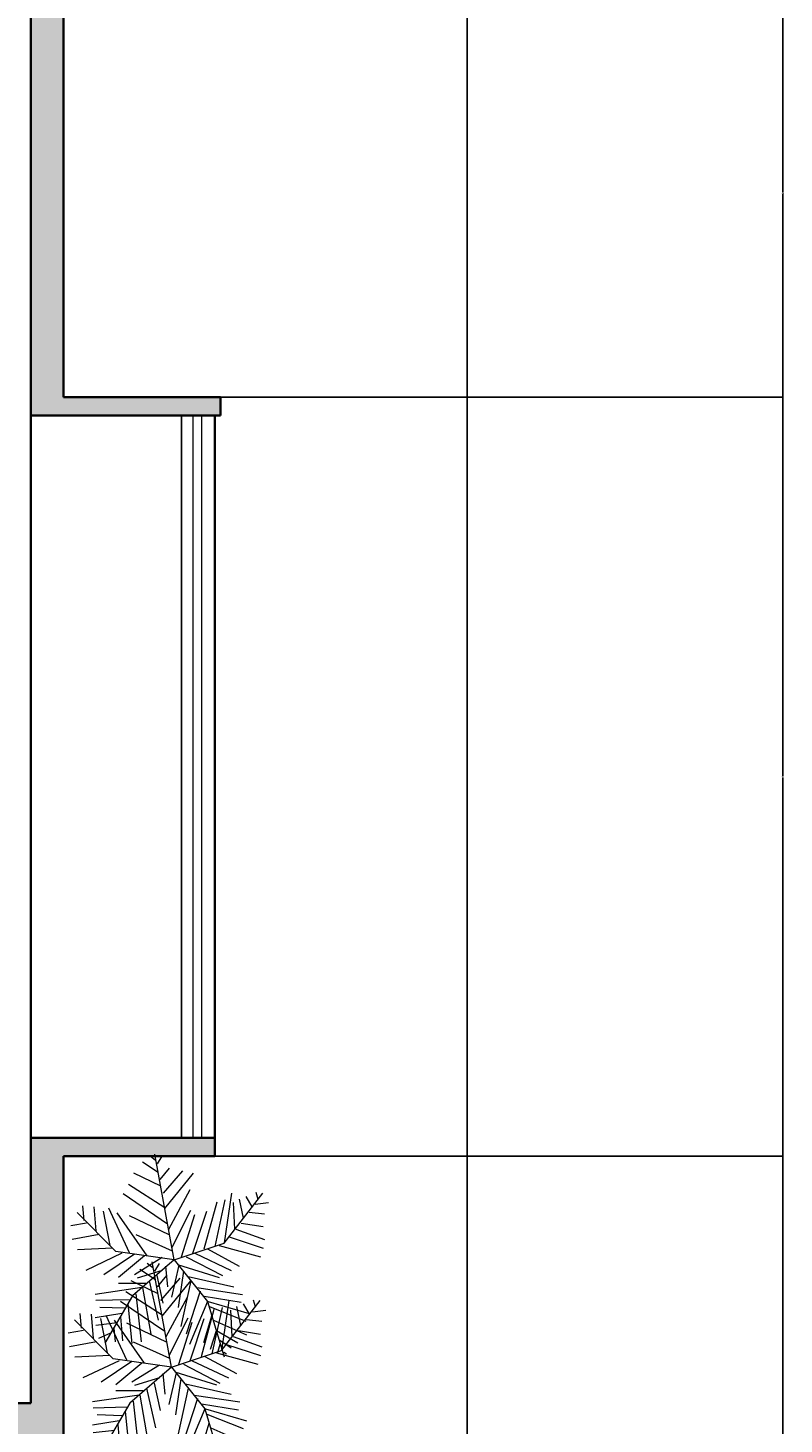
# Model space of a CAD drawing. Units: inches. Extents: x 192 to 1361, y -1362 to 367.
# Tile 22 of 23: x 1153 to 1361, y -454 to -71. Entities that reach past the tile are written whole.
import ezdxf

# ---------------------------------------------------------------- set-up
doc = ezdxf.new("R2010")
doc.units = ezdxf.units.IN
doc.header["$MEASUREMENT"] = 0
for name, color, linetype, lineweight in [('A-ANNO-DIMS', 2, 'Continuous', 18), ('A-WALL-PATT', 250, 'Continuous', 13), ('lawn', 96, 'Continuous', 13), ('walls', 7, 'Continuous', 35), ('windows', 4, 'Continuous', 18)]:
    doc.layers.add(name, color=color, linetype=linetype, lineweight=lineweight)
doc.styles.get("Standard").update_dxf_attribs({"font": 'arial.ttf'})
doc.dimstyles.get("Standard").update_dxf_attribs({"dimtxt": 0.18, "dimasz": 0.18, "dimexe": 0.18, "dimexo": 0.0625, "dimgap": 0.09, "dimtad": 0, "dimtih": 1, "dimtoh": 1, "dimzin": 0, "dimdsep": 46, "dimlunit": 3, "dimtxsty": 'Standard', "dimcen": 0.09, "dimadec": 0, "dimazin": 0, "dimtfac": 1, "dimtofl": 0, "dimtmove": 0, "dimatfit": 3, "dimfxl": 1, "dimtolj": 1, "dimtzin": 0, "dimarcsym": 0})

# ---------------------------------------------------------------- blocks, each defined once
blk = doc.blocks.new('*U4')
for p, q in [((-10.186, 53.64), (-13.084, 55.962)), ((0, 0), (-10.5, 57)), ((-9.099, 51.782), (-6.563, 55.962)), ((-7.288, 39.707), (-21.778, 46.673)), ((-8.737, 47.138), (-17.069, 52.711)), ((-7.65, 43.423), (-2.578, 49.46)), ((-5.839, 35.992), (4.667, 48.067)), ((-5.114, 27.632), (10.463, 46.673)), ((-5.114, 28.097), (-24.676, 40.636)), ((-2.941, 16.486), (8.652, 37.85)), ((-3.665, 19.273), (-27.574, 35.527)), ((16.259, 5.805), (23.142, 31.348)), ((22.055, 7.198), (27.489, 32.277)), ((27, 9), (48, 36)), ((27.127, 9.056), (31.112, 35.992)), ((31.836, 30.883), (32.561, 16.486)), ((35.096, 32.741), (37.27, 22.524)), ((38.719, 34.134), (41.979, 28.561)), ((43.791, 29.954), (51.036, 30.883)), ((44.153, 36.456), (45.239, 32.741)), ((-31.5, 4.5), (-52.5, 25.5)), ((-48.585, 21.131), (-49.309, 29.026)), ((-43.513, 28.561), (-42.427, 15.558)), ((-38.442, 26.239), (-34.819, 7.663)), ((-35.544, 28.097), (-24.314, 3.947)), ((-14.533, 2.09), (-30.834, 25.31)), ((-24.314, 23.917), (-2.941, 13.7)), ((-1.129, 6.734), (9.014, 26.704)), ((3.942, 1.625), (11.187, 24.381)), ((10.101, 3.483), (17.708, 26.239)), ((40.53, 25.775), (48.862, 24.846)), ((-47.498, 19.737), (-55.83, 18.344)), ((33.285, 16.486), (48.862, 10.913)), ((36.183, 19.737), (48.137, 17.88)), ((-40.615, 13.7), (-55.105, 10.913)), ((-20.691, 13.7), (-1.129, 4.876)), ((0, 0), (27, 9)), ((24.229, 7.663), (46.688, 1.625)), ((29.662, 12.307), (48.137, 6.269)), ((-33.37, 6.269), (-52.207, 5.34)), ((-28.299, 3.483), (-47.86, -5.805)), ((-21.416, 3.018), (-38.079, -8.128)), ((0, 0), (-31.5, 4.5)), ((-15.982, 2.09), (-30.11, -9.521)), ((0, 0), (-22.5, -19.5)), ((-6.563, 1.161), (-21.416, -8.128)), ((0, 0), (18, -22.5)), ((6.478, 1.625), (26.04, -8.592)), ((11.187, 3.483), (30.749, -5.805)), ((18.07, 5.805), (35.096, -3.483)), ((-6.563, -5.805), (-19.967, -9.985)), ((-4.752, -3.483), (-3.665, -14.629)), ((2.493, -3.019), (-1.491, -20.202)), ((1.769, -2.555), (24.229, -9.521)), ((5.029, -6.27), (2.131, -25.775)), ((-15.257, -12.772), (-30.11, -12.772)), ((-13.446, -11.378), (-8.737, -32.741)), ((-9.461, -8.592), (-6.201, -23.453)), ((9.014, -11.378), (3.58, -35.992)), ((7.565, -9.056), (32.198, -14.629)), ((-17.431, -15.094), (-42.789, -18.809)), ((-24.314, -21.596), (-42.427, -22.06)), ((-22.5, -19.5), (-37.5, -45)), ((-20.691, -18.345), (-17.793, -44.352)), ((-17.069, -15.094), (-12.721, -40.172)), ((14.085, -16.951), (6.478, -40.172)), ((18.07, -22.524), (8.289, -45.745)), ((12.274, -15.094), (36.907, -18.809)), ((16.259, -19.738), (36.183, -22.989)), ((18, -22.5), (27, -52.5)), ((18.433, -22.524), (40.53, -29.026)), ((-28.299, -29.026), (-42.789, -31.348)), ((-26.849, -26.24), (-40.253, -25.775)), ((-25.038, -23.918), (-22.865, -45.281)), ((19.157, -25.311), (38.719, -33.206)), ((-30.834, -34.135), (-42.427, -35.528)), ((-32.646, -36.921), (-31.921, -44.352)), ((-29.023, -30.884), (-27.936, -43.887)), ((20.244, -30.419), (15.897, -44.816)), ((21.331, -32.741), (39.081, -40.636)), ((-34.457, -39.708), (-40.978, -42.494)), ((22.78, -37.85), (19.519, -48.532)), ((22.78, -38.314), (34.372, -44.816)), ((24.591, -43.423), (30.749, -47.603)), ((24.591, -45.745), (23.142, -50.854)), ((26.764, -49.925), (28.213, -50.854))]:
    blk.add_line(p, q)
blk = doc.blocks.new('*D52')
at = {"layer": 'A-ANNO-DIMS', "color": 0, "lineweight": -2, "transparency": 16777216}
for p, q in [((1162.8, -60.44), (1162.8, 367.39)), ((1162.98, 367.21), (1217.73, 367.21)), ((1273.39, 367.21), (1218.64, 367.21)), ((1273.57, -597.44), (1273.57, 367.39))]:
    blk.add_line(p, q, dxfattribs=at)
at = {"layer": 'A-ANNO-DIMS', "color": 0, "transparency": 16777216}
for points in [[(1162.98, 367.24), (1162.98, 367.18), (1162.8, 367.21)], [(1273.39, 367.24), (1273.39, 367.18), (1273.57, 367.21)]]:
    blk.add_solid(points, dxfattribs=at)
at = {"layer": 'Defpoints', "color": 0, "transparency": 16777216}
for p in [(1273.57, 367.21), (1162.8, -60.5), (1273.57, -597.5)]:
    blk.add_point(p, dxfattribs=at)
at = {"layer": 'A-ANNO-DIMS', "color": 0, "transparency": 16777216, "insert": (1218.18, 367.21), "char_height": 0.18, "attachment_point": 5}
blk.add_mtext('\\A1;110.76', dxfattribs=at)
blk = doc.blocks.new('*D55')
at = {"layer": 'A-ANNO-DIMS', "color": 0, "lineweight": -2, "transparency": 16777216}
for p, q in [((1162.87, -60.5), (1360.41, -60.5)), ((1360.23, -60.68), (1360.23, -116.3)), ((1360.23, -172.29), (1360.23, -116.67)), ((1162.87, -172.47), (1360.41, -172.47))]:
    blk.add_line(p, q, dxfattribs=at)
at = {"layer": 'A-ANNO-DIMS', "color": 0, "transparency": 16777216}
for points in [[(1360.2, -60.68), (1360.26, -60.68), (1360.23, -60.5)], [(1360.2, -172.29), (1360.26, -172.29), (1360.23, -172.47)]]:
    blk.add_solid(points, dxfattribs=at)
at = {"layer": 'Defpoints', "color": 0, "transparency": 16777216}
for p in [(1162.8, -60.5), (1162.8, -172.47), (1360.23, -172.47)]:
    blk.add_point(p, dxfattribs=at)
at = {"layer": 'A-ANNO-DIMS', "color": 0, "transparency": 16777216, "insert": (1360.23, -116.49), "char_height": 0.18, "attachment_point": 5}
blk.add_mtext('\\A1;111.97', dxfattribs=at)
blk = doc.blocks.new('*D56')
at = {"layer": 'A-ANNO-DIMS', "color": 0, "lineweight": -2, "transparency": 16777216}
for p, q in [((1205.95, -172.47), (1360.41, -172.47)), ((1360.23, -172.65), (1360.23, -276.39)), ((1360.23, -380.5), (1360.23, -276.76)), ((1204.36, -380.68), (1360.41, -380.68))]:
    blk.add_line(p, q, dxfattribs=at)
at = {"layer": 'A-ANNO-DIMS', "color": 0, "transparency": 16777216}
for points in [[(1360.2, -172.65), (1360.26, -172.65), (1360.23, -172.47)], [(1360.2, -380.5), (1360.26, -380.5), (1360.23, -380.68)]]:
    blk.add_solid(points, dxfattribs=at)
at = {"layer": 'Defpoints', "color": 0, "transparency": 16777216}
for p in [(1205.89, -172.47), (1204.3, -380.68), (1360.23, -380.68)]:
    blk.add_point(p, dxfattribs=at)
at = {"layer": 'A-ANNO-DIMS', "color": 0, "transparency": 16777216, "insert": (1360.23, -276.57), "char_height": 0.18, "attachment_point": 5}
blk.add_mtext('\\A1;208.2', dxfattribs=at)
blk = doc.blocks.new('*D57')
at = {"layer": 'A-ANNO-DIMS', "color": 0, "lineweight": -2, "transparency": 16777216}
for p, q in [((1162.87, -380.68), (1360.41, -380.68)), ((1360.23, -380.86), (1360.23, -488.91)), ((1360.23, -597.32), (1360.23, -489.27)), ((1162.87, -597.5), (1360.41, -597.5))]:
    blk.add_line(p, q, dxfattribs=at)
at = {"layer": 'A-ANNO-DIMS', "color": 0, "transparency": 16777216}
for points in [[(1360.2, -380.86), (1360.26, -380.86), (1360.23, -380.68)], [(1360.2, -597.32), (1360.26, -597.32), (1360.23, -597.5)]]:
    blk.add_solid(points, dxfattribs=at)
at = {"layer": 'Defpoints', "color": 0, "transparency": 16777216}
for p in [(1162.8, -380.68), (1162.8, -597.5), (1360.23, -597.5)]:
    blk.add_point(p, dxfattribs=at)
at = {"layer": 'A-ANNO-DIMS', "color": 0, "transparency": 16777216, "insert": (1360.23, -489.09), "char_height": 0.18, "attachment_point": 5}
blk.add_mtext('\\A1;216.82', dxfattribs=at)

msp = doc.modelspace()

# ---------------------------------------------------------------- hatches: boundary and pattern name
at = {"layer": 'A-WALL-PATT'}
h = msp.add_hatch(color=256, dxfattribs=at)
h.dxf.hatch_style = 1
h.paths.add_polyline_path([(309.5452, 191.102), (300.5452, 191.102), (300.5452, -126.898), (309.5452, -126.898), (309.5452, -117.898)])
h.paths.add_polyline_path([(420.798, 191.102), (337.3229, 191.102), (337.3229, 182.102), (420.798, 182.102)])
h.paths.add_polyline_path([(518.5452, 182.102), (625.4022, 182.102), (625.4022, 191.102), (509.5452, 191.102), (509.5452, 114.3262), (518.5452, 114.3262)])
h.paths.add_polyline_path([(842.5452, 191.102), (763.4438, 191.102), (763.4438, 182.102), (833.5452, 182.102), (833.5452, 161.1615), (836.8088, 161.1615), (842.5452, 161.1615)])
h.paths.add_polyline_path([(842.5452, -16.5675), (833.5452, -16.5675), (833.5452, -60.4996), (784.8041, -60.4996), (784.8041, -354.6796), (793.8041, -354.6796), (793.8041, -69.4996), (1094.1252, -69.4996), (1094.1252, -60.4996), (842.5452, -60.4996)])
h.paths.add_polyline_path([(518.5452, 36.602), (509.5452, 36.602), (509.5452, -117.898), (420.2204, -117.898), (420.2204, -126.898), (518.5452, -126.898)])
h.paths.add_polyline_path([(474.8041, -377.0384), (465.8041, -377.0384), (465.8041, -381.5384), (465.8041, -450.898), (537.5717, -450.898), (537.5717, -441.898), (474.8041, -441.898)])
h.paths.add_polyline_path([(1162.8041, -380.6763), (1204.3001, -380.6763), (1204.3001, -375.6763), (1195.1471, -375.6763), (1153.8041, -375.6763), (1153.8041, -448.4996), (856.5691, -448.4996), (856.5691, -457.4996), (1162.8041, -457.4996)])
h.paths.add_polyline_path([(1162.8041, -525.128), (1153.8041, -525.128), (1153.8041, -597.4996), (1162.8041, -597.4996)], flags=17)
h.paths.add_polyline_path([(1162.8041, -60.4996), (1153.8041, -60.4996), (1153.8041, -69.4996), (1153.8041, -177.4733), (1205.8889, -177.4733), (1205.8889, -172.4733), (1162.8041, -172.4733)])
h.paths.add_polyline_path([(980.5799, -525.686), (971.5799, -525.686), (971.5799, -597.4996), (980.5799, -597.4996)], flags=17)
h.paths.add_polyline_path([(856.5691, -448.4996), (798.7542, -448.4996), (784.8041, -448.4996), (784.8041, -457.4996), (847.5691, -457.4996), (847.5691, -597.4996), (784.8041, -597.4996), (784.8041, -606.4996), (1273.5658, -606.4996), (1273.5658, -597.4996), (856.5691, -597.4996)])
h.paths.add_polyline_path([(1273.5658, -773.892), (1099.8366, -773.892), (1099.8366, -851.9362), (1108.8366, -851.9362), (1108.8366, -782.892), (1273.5658, -782.892)])
h.paths.add_polyline_path([(1108.8366, -982.9214), (1099.8366, -982.9214), (1099.8366, -1067.6246), (1037.7563, -1067.6246), (1037.7563, -1076.6246), (1108.8366, -1076.6246)])
h.paths.add_polyline_path([(835.078, -1067.6246), (758.8458, -1067.6246), (758.8458, -940.2324), (749.8458, -940.2324), (749.8458, -963.172), (749.8458, -970.4644), (749.8458, -1076.6246), (835.078, -1076.6246)])
h.paths.add_polyline_path([(450.307, -1066.9838), (441.307, -1066.9838), (441.307, -1076.6246), (450.307, -1076.6246)])
h.paths.add_polyline_path([(492.8925, -756.4415), (274.8925, -756.4415), (274.8925, -765.4415), (492.8925, -765.4415)])
h.paths.add_polyline_path([(283.8925, -835.2244), (274.8925, -835.2244), (274.8925, -914.4415), (492.8925, -914.4415), (492.8925, -839.9415), (483.8925, -839.9415), (483.8925, -905.4415), (283.8925, -905.4415)])
h.paths.add_polyline_path([(283.8925, -441.898), (283.8925, -375.4296), (281.6021, -375.4296), (281.6021, -399.4121), (274.8925, -399.4121), (274.8925, -441.898), (274.8925, -684.5089), (283.8925, -684.5089)])

# ---------------------------------------------------------------- linework, layer by layer
at = {"layer": 'walls'}
for p, q in [((1153.8041, -60.4996), (1153.8041, -448.4996)), ((1162.8041, -172.4733), (1162.8041, -60.4996)), ((1162.8041, -172.4733), (1205.8889, -172.4733)), ((1205.8889, -177.4733), (1205.8889, -172.4733)), ((1205.8889, -177.4733), (1153.8041, -177.4733)), ((1204.3001, -177.4733), (1204.3001, -375.6763)), ((1204.3001, -375.6763), (1153.8041, -375.6763)), ((1204.3001, -375.6763), (1204.3001, -380.6763)), ((1204.3001, -380.6763), (1162.8041, -380.6763)), ((1162.8041, -380.6763), (1162.8041, -457.4996)), ((784.8041, -448.4996), (1153.8041, -448.4996))]:
    msp.add_line(p, q, dxfattribs=at)
at = {"layer": 'windows'}
for p, q in [((1204.3001, -177.4733), (1195.1471, -177.4733)), ((1195.1471, -177.4733), (1195.1471, -375.6763)), ((1195.1471, -375.6763), (1195.1471, -177.4733)), ((1195.1471, -177.4733), (1204.3001, -177.4733)), ((1198.3483, -375.6763), (1198.3483, -177.4733)), ((1200.6621, -177.4733), (1200.6621, -375.6763)), ((1204.3001, -177.4733), (1204.3001, -375.6763)), ((1204.3001, -177.4733), (1204.3001, -375.6763)), ((1195.1471, -375.6763), (1199.6725, -375.6763)), ((1204.3001, -375.6763), (1195.1471, -375.6763)), ((1204.3001, -375.6763), (1199.6725, -375.6763))]:
    msp.add_line(p, q, dxfattribs=at)

# ---------------------------------------------------------------- block references
at = {"layer": 'lawn', "xscale": 0.5078671948952364, "yscale": 0.5078671948952364, "zscale": 0.5078671948952364}
for p in [(1193.1594, -409.106), (1192.4235, -438.5882)]:
    msp.add_blockref('*U4', p, dxfattribs=at)

# ---------------------------------------------------------------- dimensions: what is measured, and where the dimension line sits
at = {"layer": 'A-ANNO-DIMS'}
dim = msp.add_linear_dim(base=(1273.5658, 367.2097), p1=(1162.8041, -60.4996), p2=(1273.5658, -597.4996), dimstyle='Standard', override={"dimdec": 2, "dimlfac": 1, "dimrnd": 0, "dimzin": 0, "dimdsep": 46, "dimlunit": 2}, dxfattribs=at)
dim.commit()
dim.dimension.update_dxf_attribs({"geometry": '*D52', "text_midpoint": (1218.185, 367.2097)})
for base, p1, p2, override, picture, middle in [((1360.2331, -172.4733), (1162.8041, -60.4996), (1162.8041, -172.4733), {"dimdec": 2, "dimlfac": 1, "dimrnd": 0, "dimzin": 0, "dimdsep": 46, "dimlunit": 2}, '*D55', (1360.2331, -116.4864)), ((1360.2331, -380.6763), (1205.8889, -172.4733), (1204.3001, -380.6763), {"dimdec": 1, "dimlfac": 1, "dimrnd": 0, "dimzin": 0, "dimdsep": 46, "dimlunit": 2}, '*D56', (1360.2331, -276.5748)), ((1360.2331, -597.4996), (1162.8041, -380.6763), (1162.8041, -597.4996), {"dimdec": 2, "dimlfac": 1, "dimrnd": 0, "dimzin": 0, "dimdsep": 46, "dimlunit": 2}, '*D57', (1360.2331, -489.0879))]:
    dim = msp.add_linear_dim(base=base, p1=p1, p2=p2, angle=90, dimstyle='Standard', override=override, dxfattribs=at)
    dim.commit()
    dim.dimension.update_dxf_attribs({"geometry": picture, "text_midpoint": middle})

doc.saveas('drawing.dxf')
